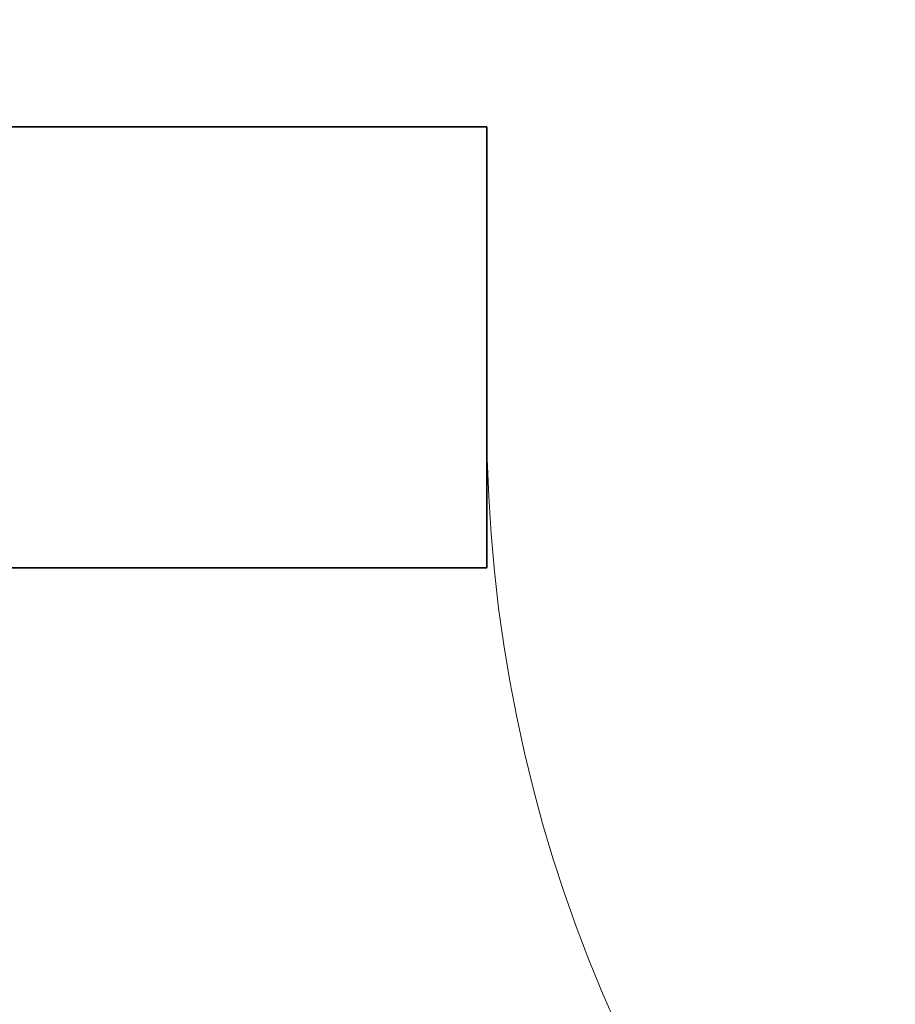
# Model space of a CAD drawing. Units: inches. Extents: x 3321 to 5237, y 11 to 1752.
# Tile 33 of 43: x 5077.55 to 5095.42, y 1416.43 to 1436.52. Entities that reach past the tile are written whole.
import ezdxf

# ---------------------------------------------------------------- set-up
doc = ezdxf.new("R2010")
doc.units = ezdxf.units.IN
for name, color, linetype, lineweight in [('A-ANNO-DIMS', 2, 'Continuous', 18), ('A-DOOR', 4, 'Continuous', 18), ('A-WALL', 7, 'Continuous', 35)]:
    doc.layers.add(name, color=color, linetype=linetype, lineweight=lineweight)
doc.styles.get("Standard").update_dxf_attribs({"font": 'arial.ttf'})
doc.dimstyles.new('ISO-25', dxfattribs={"dimtxt": 9, "dimasz": 2.5, "dimexe": 1.25, "dimexo": 0.625, "dimtad": 1, "dimdec": 1, "dimlunit": 3, "dimtxsty": 'Standard', "dimcen": 2.5, "dimclrd": 4, "dimclre": 4, "dimclrt": 256, "dimadec": 0, "dimazin": 0, "dimtfac": 1, "dimtdec": 1, "dimtmove": 0, "dimatfit": 3, "dimfxl": 1, "dimarcsym": 0})

# ---------------------------------------------------------------- blocks, each defined once
blk = doc.blocks.new('*U8')
blk.add_line((-30, 0), (-30, 6))
blk.add_arc((0, 0), 30, 180, 270)
blk = doc.blocks.new('*D194')
at = {"layer": 'A-ANNO-DIMS', "color": 4, "lineweight": -2, "transparency": 16777216}
for p, q in [((5037.321, 1452.516), (5037.321, 1436.712)), ((5121.084, 1452.516), (5121.084, 1436.712)), ((5039.821, 1437.962), (5118.584, 1437.962))]:
    blk.add_line(p, q, dxfattribs=at)
at = {"layer": 'A-ANNO-DIMS', "color": 4, "transparency": 16777216}
for points in [[(5039.821, 1438.379), (5039.821, 1437.545), (5037.321, 1437.962)], [(5118.584, 1438.379), (5118.584, 1437.545), (5121.084, 1437.962)]]:
    blk.add_solid(points, dxfattribs=at)
at = {"layer": 'Defpoints', "color": 0, "transparency": 16777216}
for p in [(5037.321, 1453.141), (5121.084, 1453.141), (5121.084, 1437.962)]:
    blk.add_point(p, dxfattribs=at)
at = {"layer": 'A-ANNO-DIMS', "transparency": 16777216, "insert": (5079.203, 1443.182), "char_height": 9, "attachment_point": 5}
blk.add_mtext('7\'-0" TYP.', dxfattribs=at)
blk = doc.blocks.new('*D197')
at = {"layer": 'A-ANNO-DIMS', "color": 4, "lineweight": -2, "transparency": 16777216}
for p, q in [((5117.009, 1364.83), (5117.009, 1476.212)), ((5114.11, 1364.83), (5118.259, 1364.83)), ((5117.009, 1343.839), (5117.009, 1362.33)), ((5114.11, 1341.339), (5118.259, 1341.339))]:
    blk.add_line(p, q, dxfattribs=at)
at = {"layer": 'A-ANNO-DIMS', "color": 4, "transparency": 16777216}
for points in [[(5116.592, 1362.33), (5117.426, 1362.33), (5117.009, 1364.83)], [(5116.592, 1343.839), (5117.426, 1343.839), (5117.009, 1341.339)]]:
    blk.add_solid(points, dxfattribs=at)
at = {"layer": 'Defpoints', "color": 0, "transparency": 16777216}
for p in [(5113.485, 1364.83), (5117.009, 1364.83), (5113.485, 1341.339)]:
    blk.add_point(p, dxfattribs=at)
at = {"layer": 'A-ANNO-DIMS', "transparency": 16777216, "insert": (5111.731, 1421.771), "char_height": 9, "attachment_point": 5, "rotation": 90}
blk.add_mtext('WC 1\'-11 1/2" TYP.', dxfattribs=at)

msp = doc.modelspace()

# ---------------------------------------------------------------- linework, layer by layer
at = {"layer": 'A-WALL'}
for p, q in [((5001.084, 1434.339), (5087.084, 1434.339)), ((5087.084, 1434.339), (5087.084, 1425.339)), ((5061.084, 1425.339), (5087.084, 1425.339))]:
    msp.add_line(p, q, dxfattribs=at)

# ---------------------------------------------------------------- block references
at = {"layer": 'A-DOOR'}
msp.add_blockref('*U8', (5117.084, 1428.339), dxfattribs=at)

# ---------------------------------------------------------------- dimensions: what is measured, and where the dimension line sits
at = {"layer": 'A-ANNO-DIMS'}
dim = msp.add_linear_dim(base=(5117.009, 1364.83), p1=(5113.485, 1341.339), p2=(5113.485, 1364.83), angle=90, text='WC <> TYP.', dimstyle='ISO-25', override={"dimdec": 1, "dimlfac": 1, "dimrnd": 0, "dimzin": 1, "dimdsep": 46, "dimlunit": 4, "dimfrac": 2}, dxfattribs=at)
dim.commit()
dim.dimension.update_dxf_attribs({"geometry": '*D197', "text_midpoint": (5111.731, 1421.771)})
dim = msp.add_linear_dim(base=(5121.084, 1437.962), p1=(5037.321, 1453.141), p2=(5121.084, 1453.141), text='<> TYP.', dimstyle='ISO-25', override={"dimdec": 1, "dimlfac": 1, "dimrnd": 0, "dimzin": 1, "dimdsep": 46, "dimlunit": 4, "dimfrac": 2}, dxfattribs=at)
dim.commit()
dim.dimension.update_dxf_attribs({"geometry": '*D194', "text_midpoint": (5079.203, 1443.182)})

doc.saveas('drawing.dxf')
